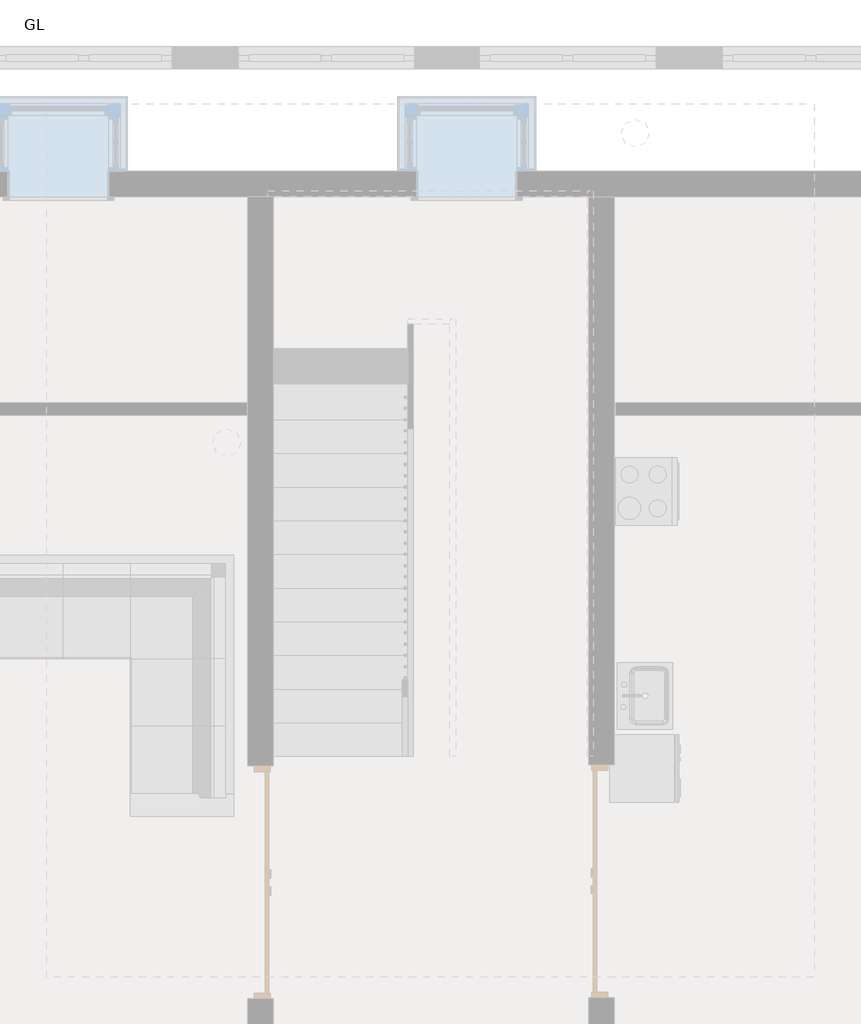
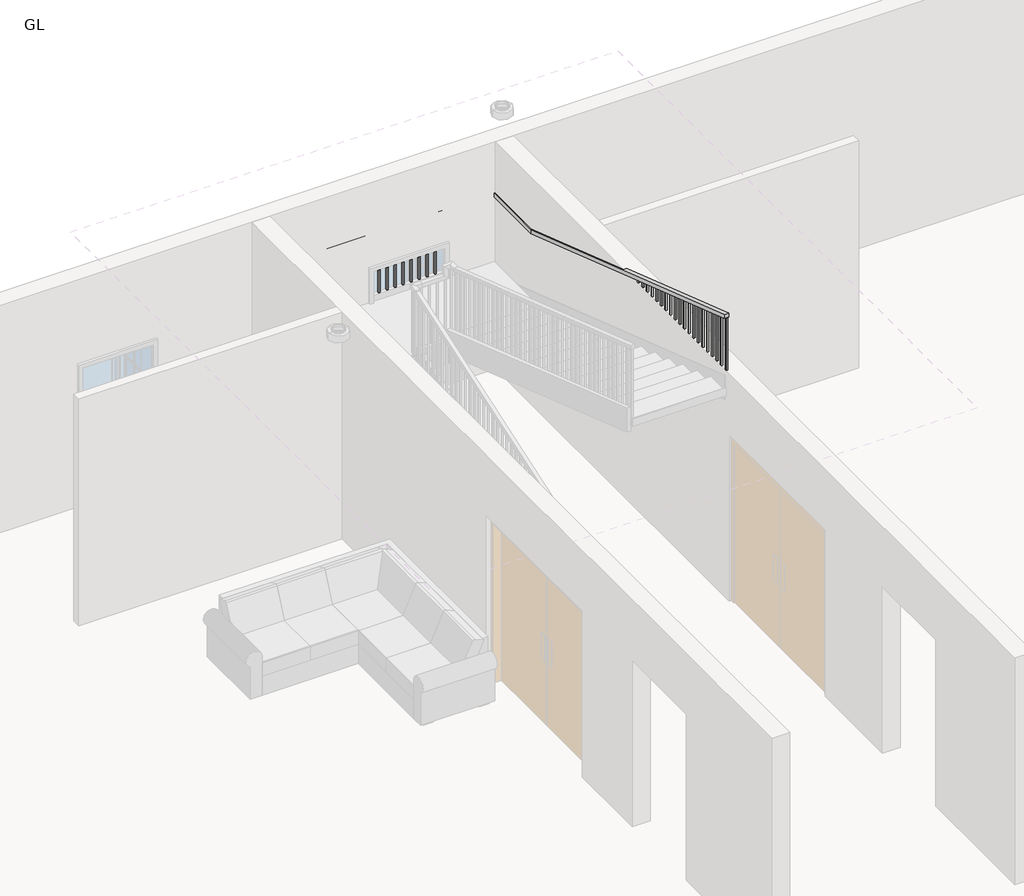
# One storey, part 3 of 5: 1 railing.
"""IFC4 building model written with IfcOpenShell, lengths in millimetres."""

from ifc_helpers import new_model, si_unit, frame, origin, place, context, project, spatial, polyline, outline, extrude, faceted_brep, element, save

model = new_model("IFC4")

# Units and contexts
model_context = context("Model", 3, world=origin())
ifc_project = project(units=[si_unit("LENGTHUNIT", "METRE", prefix="MILLI")], contexts=[model_context])

# Site, building, storey
site = spatial("IfcSite", under=ifc_project)
building = spatial("IfcBuilding", under=site)
storey = spatial("IfcBuildingStorey", under=building, Name="GL", Elevation=0.0)

# Railing
placement = place(None, origin())
element("IfcRailing", 1, ObjectType="Handrail - Rectangular", at=placement, inside=storey, context=model_context, shape_type="SolidModel", body=[
    faceted_brep([(-1899.5987998, 2564.5067329, 1017.8142857), (-1899.5987998, 2564.5067329, 964.1699957), (-1848.7987998, 2564.5067329, 964.1699957), (-1848.7987998, 2564.5067329, 1017.8142857), (-1899.5987998, 6526.9067329, 2362.2), (-1899.5987998, 6535.2899033, 2311.4), (-1848.7987998, 6535.2899033, 2311.4), (-1848.7987998, 6526.9067329, 2362.2), (-1899.5987998, 7682.6067329, 2311.4), (-1899.5987998, 7682.6067329, 2362.2), (1046.8012002, 7682.6067329, 2362.2), (1046.8012002, 7682.6067329, 2311.4), (-1848.7987998, 7631.8067329, 2311.4), (996.0012002, 7631.8067329, 2311.4), (-1848.7987998, 7631.8067329, 2362.2), (996.0012002, 7631.8067329, 2362.2), (1046.8012002, 6831.7067329, 2362.2), (1046.8012002, 6823.3235624, 2311.4), (996.0012002, 6823.3235624, 2311.4), (996.0012002, 6831.7067329, 2362.2), (1046.8012002, 2564.5067329, 3810.0), (996.0012002, 2564.5067329, 3810.0), (996.0012002, 2564.5067329, 3756.35571), (1046.8012002, 2564.5067329, 3756.35571)], [[[0, 1, 2, 3]], [[1, 0, 4, 5]], [[2, 1, 5, 6]], [[3, 2, 6, 7]], [[0, 3, 7, 4]], [[8, 9, 10, 11]], [[12, 8, 11, 13]], [[14, 12, 13, 15]], [[9, 14, 15, 10]], [[11, 10, 16, 17]], [[13, 11, 17, 18]], [[15, 13, 18, 19]], [[10, 15, 19, 16]], [[5, 4, 9, 8]], [[6, 5, 8, 12]], [[7, 6, 12, 14]], [[4, 7, 14, 9]], [[20, 21, 22, 23]], [[17, 16, 20, 23]], [[18, 17, 23, 22]], [[19, 18, 22, 21]], [[16, 19, 21, 20]]]),
    extrude(outline(polyline([(2586.7317329, 3748.815085), (2586.7317329, 2977.8831452), (2567.6817329, 2984.3465381), (2567.6817329, 3755.2784779), (2586.7317329, 3748.815085)])), frame((1011.8762002, 0.0, 0.0), z_axis=(1.0, 0.0, 0.0), x_axis=(0.0, 1.0, 0.0)), (0.0, 0.0, 1.0), 19.05),
    extrude(outline(polyline([(2688.3317329, 3714.3436565), (2688.3317329, 2943.4117167), (2669.2817329, 2949.8751095), (2669.2817329, 3720.8070493), (2688.3317329, 3714.3436565)])), frame((1011.8762002, 0.0, 0.0), z_axis=(1.0, 0.0, 0.0), x_axis=(0.0, 1.0, 0.0)), (0.0, 0.0, 1.0), 19.05),
    extrude(outline(polyline([(2789.9317329, 3679.8722279), (2789.9317329, 2908.9402881), (2770.8817329, 2915.403681), (2770.8817329, 3686.3356207), (2789.9317329, 3679.8722279)])), frame((1011.8762002, 0.0, 0.0), z_axis=(1.0, 0.0, 0.0), x_axis=(0.0, 1.0, 0.0)), (0.0, 0.0, 1.0), 19.05),
    extrude(outline(polyline([(2891.5317329, 3645.4007993), (2891.5317329, 2874.4688595), (2872.4817329, 2880.9322524), (2872.4817329, 3651.8641922), (2891.5317329, 3645.4007993)])), frame((1011.8762002, 0.0, 0.0), z_axis=(1.0, 0.0, 0.0), x_axis=(0.0, 1.0, 0.0)), (0.0, 0.0, 1.0), 19.05),
    extrude(outline(polyline([(2993.1317329, 3610.9293707), (2993.1317329, 2839.997431), (2974.0817329, 2846.4608238), (2974.0817329, 3617.3927636), (2993.1317329, 3610.9293707)])), frame((1011.8762002, 0.0, 0.0), z_axis=(1.0, 0.0, 0.0), x_axis=(0.0, 1.0, 0.0)), (0.0, 0.0, 1.0), 19.05),
    extrude(outline(polyline([(3094.7317329, 3576.4579422), (3094.7317329, 2805.5260024), (3075.6817329, 2811.9893952), (3075.6817329, 3582.921335), (3094.7317329, 3576.4579422)])), frame((1011.8762002, 0.0, 0.0), z_axis=(1.0, 0.0, 0.0), x_axis=(0.0, 1.0, 0.0)), (0.0, 0.0, 1.0), 19.05),
    extrude(outline(polyline([(3196.3317329, 3541.9865136), (3196.3317329, 2771.0545738), (3177.2817329, 2777.5179667), (3177.2817329, 3548.4499065), (3196.3317329, 3541.9865136)])), frame((1011.8762002, 0.0, 0.0), z_axis=(1.0, 0.0, 0.0), x_axis=(0.0, 1.0, 0.0)), (0.0, 0.0, 1.0), 19.05),
    extrude(outline(polyline([(3297.9317329, 3507.515085), (3297.9317329, 2736.5831452), (3278.8817329, 2743.0465381), (3278.8817329, 3513.9784779), (3297.9317329, 3507.515085)])), frame((1011.8762002, 0.0, 0.0), z_axis=(1.0, 0.0, 0.0), x_axis=(0.0, 1.0, 0.0)), (0.0, 0.0, 1.0), 19.05),
    extrude(outline(polyline([(3399.5317329, 3473.0436565), (3399.5317329, 2702.1117167), (3380.4817329, 2708.5751095), (3380.4817329, 3479.5070493), (3399.5317329, 3473.0436565)])), frame((1011.8762002, 0.0, 0.0), z_axis=(1.0, 0.0, 0.0), x_axis=(0.0, 1.0, 0.0)), (0.0, 0.0, 1.0), 19.05),
    extrude(outline(polyline([(3501.1317329, 3438.5722279), (3501.1317329, 2667.6402881), (3482.0817329, 2674.103681), (3482.0817329, 3445.0356207), (3501.1317329, 3438.5722279)])), frame((1011.8762002, 0.0, 0.0), z_axis=(1.0, 0.0, 0.0), x_axis=(0.0, 1.0, 0.0)), (0.0, 0.0, 1.0), 19.05),
    extrude(outline(polyline([(3602.7317329, 3404.1007993), (3602.7317329, 2633.1688595), (3583.6817329, 2639.6322524), (3583.6817329, 3410.5641922), (3602.7317329, 3404.1007993)])), frame((1011.8762002, 0.0, 0.0), z_axis=(1.0, 0.0, 0.0), x_axis=(0.0, 1.0, 0.0)), (0.0, 0.0, 1.0), 19.05),
    extrude(outline(polyline([(3704.3317329, 3369.6293707), (3704.3317329, 2598.697431), (3685.2817329, 2605.1608238), (3685.2817329, 3376.0927636), (3704.3317329, 3369.6293707)])), frame((1011.8762002, 0.0, 0.0), z_axis=(1.0, 0.0, 0.0), x_axis=(0.0, 1.0, 0.0)), (0.0, 0.0, 1.0), 19.05),
    extrude(outline(polyline([(3805.9317329, 3335.1579422), (3805.9317329, 2564.2260024), (3786.8817329, 2570.6893952), (3786.8817329, 3341.621335), (3805.9317329, 3335.1579422)])), frame((1011.8762002, 0.0, 0.0), z_axis=(1.0, 0.0, 0.0), x_axis=(0.0, 1.0, 0.0)), (0.0, 0.0, 1.0), 19.05),
    extrude(outline(polyline([(3907.5317329, 3300.6865136), (3907.5317329, 2529.7545738), (3888.4817329, 2536.2179667), (3888.4817329, 3307.1499065), (3907.5317329, 3300.6865136)])), frame((1011.8762002, 0.0, 0.0), z_axis=(1.0, 0.0, 0.0), x_axis=(0.0, 1.0, 0.0)), (0.0, 0.0, 1.0), 19.05),
    extrude(outline(polyline([(4009.1317329, 3266.215085), (4009.1317329, 2495.2831452), (3990.0817329, 2501.7465381), (3990.0817329, 3272.6784779), (4009.1317329, 3266.215085)])), frame((1011.8762002, 0.0, 0.0), z_axis=(1.0, 0.0, 0.0), x_axis=(0.0, 1.0, 0.0)), (0.0, 0.0, 1.0), 19.05),
    extrude(outline(polyline([(4110.7317329, 3231.7436565), (4110.7317329, 2460.8117167), (4091.6817329, 2467.2751095), (4091.6817329, 3238.2070493), (4110.7317329, 3231.7436565)])), frame((1011.8762002, 0.0, 0.0), z_axis=(1.0, 0.0, 0.0), x_axis=(0.0, 1.0, 0.0)), (0.0, 0.0, 1.0), 19.05),
    extrude(outline(polyline([(4212.3317329, 3197.2722279), (4212.3317329, 2426.3402881), (4193.2817329, 2432.803681), (4193.2817329, 3203.7356207), (4212.3317329, 3197.2722279)])), frame((1011.8762002, 0.0, 0.0), z_axis=(1.0, 0.0, 0.0), x_axis=(0.0, 1.0, 0.0)), (0.0, 0.0, 1.0), 19.05),
    extrude(outline(polyline([(4313.9317329, 3162.8007993), (4313.9317329, 2391.8688595), (4294.8817329, 2398.3322524), (4294.8817329, 3169.2641922), (4313.9317329, 3162.8007993)])), frame((1011.8762002, 0.0, 0.0), z_axis=(1.0, 0.0, 0.0), x_axis=(0.0, 1.0, 0.0)), (0.0, 0.0, 1.0), 19.05),
    extrude(outline(polyline([(4415.5317329, 3128.3293707), (4415.5317329, 2357.397431), (4396.4817329, 2363.8608238), (4396.4817329, 3134.7927636), (4415.5317329, 3128.3293707)])), frame((1011.8762002, 0.0, 0.0), z_axis=(1.0, 0.0, 0.0), x_axis=(0.0, 1.0, 0.0)), (0.0, 0.0, 1.0), 19.05),
    extrude(outline(polyline([(4517.1317329, 3093.8579422), (4517.1317329, 2322.9260024), (4498.0817329, 2329.3893952), (4498.0817329, 3100.321335), (4517.1317329, 3093.8579422)])), frame((1011.8762002, 0.0, 0.0), z_axis=(1.0, 0.0, 0.0), x_axis=(0.0, 1.0, 0.0)), (0.0, 0.0, 1.0), 19.05),
    extrude(outline(polyline([(4618.7317329, 3059.3865136), (4618.7317329, 2288.4545738), (4599.6817329, 2294.9179667), (4599.6817329, 3065.8499065), (4618.7317329, 3059.3865136)])), frame((1011.8762002, 0.0, 0.0), z_axis=(1.0, 0.0, 0.0), x_axis=(0.0, 1.0, 0.0)), (0.0, 0.0, 1.0), 19.05),
    extrude(outline(polyline([(4720.3317329, 3024.915085), (4720.3317329, 2253.9831452), (4701.2817329, 2260.4465381), (4701.2817329, 3031.3784779), (4720.3317329, 3024.915085)])), frame((1011.8762002, 0.0, 0.0), z_axis=(1.0, 0.0, 0.0), x_axis=(0.0, 1.0, 0.0)), (0.0, 0.0, 1.0), 19.05),
    extrude(outline(polyline([(4821.9317329, 2990.4436565), (4821.9317329, 2219.5117167), (4802.8817329, 2225.9751095), (4802.8817329, 2996.9070493), (4821.9317329, 2990.4436565)])), frame((1011.8762002, 0.0, 0.0), z_axis=(1.0, 0.0, 0.0), x_axis=(0.0, 1.0, 0.0)), (0.0, 0.0, 1.0), 19.05),
    extrude(outline(polyline([(4923.5317329, 2955.9722279), (4923.5317329, 2185.0402881), (4904.4817329, 2191.503681), (4904.4817329, 2962.4356207), (4923.5317329, 2955.9722279)])), frame((1011.8762002, 0.0, 0.0), z_axis=(1.0, 0.0, 0.0), x_axis=(0.0, 1.0, 0.0)), (0.0, 0.0, 1.0), 19.05),
    extrude(outline(polyline([(5025.1317329, 2921.5007993), (5025.1317329, 2150.5688595), (5006.0817329, 2157.0322524), (5006.0817329, 2927.9641922), (5025.1317329, 2921.5007993)])), frame((1011.8762002, 0.0, 0.0), z_axis=(1.0, 0.0, 0.0), x_axis=(0.0, 1.0, 0.0)), (0.0, 0.0, 1.0), 19.05),
    extrude(outline(polyline([(5126.7317329, 2887.0293707), (5126.7317329, 2116.097431), (5107.6817329, 2122.5608238), (5107.6817329, 2893.4927636), (5126.7317329, 2887.0293707)])), frame((1011.8762002, 0.0, 0.0), z_axis=(1.0, 0.0, 0.0), x_axis=(0.0, 1.0, 0.0)), (0.0, 0.0, 1.0), 19.05),
    extrude(outline(polyline([(5228.3317329, 2852.5579422), (5228.3317329, 2081.6260024), (5209.2817329, 2088.0893952), (5209.2817329, 2859.021335), (5228.3317329, 2852.5579422)])), frame((1011.8762002, 0.0, 0.0), z_axis=(1.0, 0.0, 0.0), x_axis=(0.0, 1.0, 0.0)), (0.0, 0.0, 1.0), 19.05),
    extrude(outline(polyline([(5329.9317329, 2818.0865136), (5329.9317329, 2047.1545738), (5310.8817329, 2053.6179667), (5310.8817329, 2824.5499065), (5329.9317329, 2818.0865136)])), frame((1011.8762002, 0.0, 0.0), z_axis=(1.0, 0.0, 0.0), x_axis=(0.0, 1.0, 0.0)), (0.0, 0.0, 1.0), 19.05),
    extrude(outline(polyline([(5431.5317329, 2783.615085), (5431.5317329, 2012.6831452), (5412.4817329, 2019.1465381), (5412.4817329, 2790.0784779), (5431.5317329, 2783.615085)])), frame((1011.8762002, 0.0, 0.0), z_axis=(1.0, 0.0, 0.0), x_axis=(0.0, 1.0, 0.0)), (0.0, 0.0, 1.0), 19.05),
    extrude(outline(polyline([(5533.1317329, 2749.1436565), (5533.1317329, 1978.2117167), (5514.0817329, 1984.6751095), (5514.0817329, 2755.6070493), (5533.1317329, 2749.1436565)])), frame((1011.8762002, 0.0, 0.0), z_axis=(1.0, 0.0, 0.0), x_axis=(0.0, 1.0, 0.0)), (0.0, 0.0, 1.0), 19.05),
    extrude(outline(polyline([(5634.7317329, 2714.6722279), (5634.7317329, 1943.7402881), (5615.6817329, 1950.203681), (5615.6817329, 2721.1356207), (5634.7317329, 2714.6722279)])), frame((1011.8762002, 0.0, 0.0), z_axis=(1.0, 0.0, 0.0), x_axis=(0.0, 1.0, 0.0)), (0.0, 0.0, 1.0), 19.05),
    extrude(outline(polyline([(5736.3317329, 2680.2007993), (5736.3317329, 1909.2688595), (5717.2817329, 1915.7322524), (5717.2817329, 2686.6641922), (5736.3317329, 2680.2007993)])), frame((1011.8762002, 0.0, 0.0), z_axis=(1.0, 0.0, 0.0), x_axis=(0.0, 1.0, 0.0)), (0.0, 0.0, 1.0), 19.05),
    extrude(outline(polyline([(5837.9317329, 2645.7293707), (5837.9317329, 1874.797431), (5818.8817329, 1881.2608238), (5818.8817329, 2652.1927636), (5837.9317329, 2645.7293707)])), frame((1011.8762002, 0.0, 0.0), z_axis=(1.0, 0.0, 0.0), x_axis=(0.0, 1.0, 0.0)), (0.0, 0.0, 1.0), 19.05),
    extrude(outline(polyline([(5939.5317329, 2611.2579422), (5939.5317329, 1840.3260024), (5920.4817329, 1846.7893952), (5920.4817329, 2617.721335), (5939.5317329, 2611.2579422)])), frame((1011.8762002, 0.0, 0.0), z_axis=(1.0, 0.0, 0.0), x_axis=(0.0, 1.0, 0.0)), (0.0, 0.0, 1.0), 19.05),
    extrude(outline(polyline([(6041.1317329, 2576.7865136), (6041.1317329, 1805.8545738), (6022.0817329, 1812.3179667), (6022.0817329, 2583.2499065), (6041.1317329, 2576.7865136)])), frame((1011.8762002, 0.0, 0.0), z_axis=(1.0, 0.0, 0.0), x_axis=(0.0, 1.0, 0.0)), (0.0, 0.0, 1.0), 19.05),
    extrude(outline(polyline([(6142.7317329, 2542.315085), (6142.7317329, 1771.3831452), (6123.6817329, 1777.8465381), (6123.6817329, 2548.7784779), (6142.7317329, 2542.315085)])), frame((1011.8762002, 0.0, 0.0), z_axis=(1.0, 0.0, 0.0), x_axis=(0.0, 1.0, 0.0)), (0.0, 0.0, 1.0), 19.05),
    extrude(outline(polyline([(6244.3317329, 2507.8436565), (6244.3317329, 1736.9117167), (6225.2817329, 1743.3751095), (6225.2817329, 2514.3070493), (6244.3317329, 2507.8436565)])), frame((1011.8762002, 0.0, 0.0), z_axis=(1.0, 0.0, 0.0), x_axis=(0.0, 1.0, 0.0)), (0.0, 0.0, 1.0), 19.05),
    extrude(outline(polyline([(6345.9317329, 2473.3722279), (6345.9317329, 1702.4402881), (6326.8817329, 1708.903681), (6326.8817329, 2479.8356207), (6345.9317329, 2473.3722279)])), frame((1011.8762002, 0.0, 0.0), z_axis=(1.0, 0.0, 0.0), x_axis=(0.0, 1.0, 0.0)), (0.0, 0.0, 1.0), 19.05),
    extrude(outline(polyline([(6447.5317329, 2438.9007993), (6447.5317329, 1667.9688595), (6428.4817329, 1674.4322524), (6428.4817329, 2445.3641922), (6447.5317329, 2438.9007993)])), frame((1011.8762002, 0.0, 0.0), z_axis=(1.0, 0.0, 0.0), x_axis=(0.0, 1.0, 0.0)), (0.0, 0.0, 1.0), 19.05),
    extrude(outline(polyline([(6549.1317329, 2404.4293707), (6549.1317329, 1633.497431), (6530.0817329, 1639.9608238), (6530.0817329, 2410.8927636), (6549.1317329, 2404.4293707)])), frame((1011.8762002, 0.0, 0.0), z_axis=(1.0, 0.0, 0.0), x_axis=(0.0, 1.0, 0.0)), (0.0, 0.0, 1.0), 19.05),
    extrude(outline(polyline([(6650.7317329, 2369.9579422), (6650.7317329, 1599.0260024), (6631.6817329, 1605.4893952), (6631.6817329, 2376.421335), (6650.7317329, 2369.9579422)])), frame((1011.8762002, 0.0, 0.0), z_axis=(1.0, 0.0, 0.0), x_axis=(0.0, 1.0, 0.0)), (0.0, 0.0, 1.0), 19.05),
    extrude(outline(polyline([(6752.3317329, 2335.4865136), (6752.3317329, 1564.5545738), (6733.2817329, 1571.0179667), (6733.2817329, 2341.9499065), (6752.3317329, 2335.4865136)])), frame((1011.8762002, 0.0, 0.0), z_axis=(1.0, 0.0, 0.0), x_axis=(0.0, 1.0, 0.0)), (0.0, 0.0, 1.0), 19.05),
    extrude(outline(polyline([(6853.9317329, 2311.4), (6853.9317329, 1530.0831452), (6834.8817329, 1536.5465381), (6834.8817329, 2311.4), (6853.9317329, 2311.4)])), frame((1011.8762002, 0.0, 0.0), z_axis=(1.0, 0.0, 0.0), x_axis=(0.0, 1.0, 0.0)), (0.0, 0.0, 1.0), 19.05),
    extrude(outline(polyline([(6955.5317329, 2311.4), (6955.5317329, 1495.6117167), (6936.4817329, 1502.0751095), (6936.4817329, 2311.4), (6955.5317329, 2311.4)])), frame((1011.8762002, 0.0, 0.0), z_axis=(1.0, 0.0, 0.0), x_axis=(0.0, 1.0, 0.0)), (0.0, 0.0, 1.0), 19.05),
    extrude(outline(polyline([(7057.1317329, 2311.4), (7057.1317329, 1461.1402881), (7038.0817329, 1467.603681), (7038.0817329, 2311.4), (7057.1317329, 2311.4)])), frame((1011.8762002, 0.0, 0.0), z_axis=(1.0, 0.0, 0.0), x_axis=(0.0, 1.0, 0.0)), (0.0, 0.0, 1.0), 19.05),
    extrude(outline(polyline([(7158.7317329, 2311.4), (7158.7317329, 1426.6688595), (7139.6817329, 1433.1322524), (7139.6817329, 2311.4), (7158.7317329, 2311.4)])), frame((1011.8762002, 0.0, 0.0), z_axis=(1.0, 0.0, 0.0), x_axis=(0.0, 1.0, 0.0)), (0.0, 0.0, 1.0), 19.05),
    extrude(outline(polyline([(7260.3317329, 2311.4), (7260.3317329, 1392.197431), (7241.2817329, 1398.6608238), (7241.2817329, 2311.4), (7260.3317329, 2311.4)])), frame((1011.8762002, 0.0, 0.0), z_axis=(1.0, 0.0, 0.0), x_axis=(0.0, 1.0, 0.0)), (0.0, 0.0, 1.0), 19.05),
    extrude(outline(polyline([(7361.9317329, 2311.4), (7361.9317329, 1357.7260024), (7342.8817329, 1364.1893952), (7342.8817329, 2311.4), (7361.9317329, 2311.4)])), frame((1011.8762002, 0.0, 0.0), z_axis=(1.0, 0.0, 0.0), x_axis=(0.0, 1.0, 0.0)), (0.0, 0.0, 1.0), 19.05),
    extrude(outline(polyline([(7463.5317329, 2311.4), (7463.5317329, 1323.2545738), (7444.4817329, 1329.7179667), (7444.4817329, 2311.4), (7463.5317329, 2311.4)])), frame((1011.8762002, 0.0, 0.0), z_axis=(1.0, 0.0, 0.0), x_axis=(0.0, 1.0, 0.0)), (0.0, 0.0, 1.0), 19.05),
    extrude(outline(polyline([(7565.1317329, 2311.4), (7565.1317329, 1288.7831452), (7546.0817329, 1295.2465381), (7546.0817329, 2311.4), (7565.1317329, 2311.4)])), frame((1011.8762002, 0.0, 0.0), z_axis=(1.0, 0.0, 0.0), x_axis=(0.0, 1.0, 0.0)), (0.0, 0.0, 1.0), 19.05),
    extrude(outline(polyline([(961.0762002, 7666.7317329), (980.1262002, 7666.7317329), (980.1262002, 7647.6817329), (961.0762002, 7647.6817329), (961.0762002, 7666.7317329)])), frame((0.0, 0.0, 1524.0), z_axis=(0.0, 0.0, 1.0), x_axis=(1.0, 0.0, 0.0)), (0.0, 0.0, 1.0), 787.4),
    extrude(outline(polyline([(859.4762002, 7666.7317329), (878.5262002, 7666.7317329), (878.5262002, 7647.6817329), (859.4762002, 7647.6817329), (859.4762002, 7666.7317329)])), frame((0.0, 0.0, 1524.0), z_axis=(0.0, 0.0, 1.0), x_axis=(1.0, 0.0, 0.0)), (0.0, 0.0, 1.0), 787.4),
    extrude(outline(polyline([(757.8762002, 7666.7317329), (776.9262002, 7666.7317329), (776.9262002, 7647.6817329), (757.8762002, 7647.6817329), (757.8762002, 7666.7317329)])), frame((0.0, 0.0, 1524.0), z_axis=(0.0, 0.0, 1.0), x_axis=(1.0, 0.0, 0.0)), (0.0, 0.0, 1.0), 787.4),
    extrude(outline(polyline([(656.2762002, 7666.7317329), (675.3262002, 7666.7317329), (675.3262002, 7647.6817329), (656.2762002, 7647.6817329), (656.2762002, 7666.7317329)])), frame((0.0, 0.0, 1524.0), z_axis=(0.0, 0.0, 1.0), x_axis=(1.0, 0.0, 0.0)), (0.0, 0.0, 1.0), 787.4),
    extrude(outline(polyline([(554.6762002, 7666.7317329), (573.7262002, 7666.7317329), (573.7262002, 7647.6817329), (554.6762002, 7647.6817329), (554.6762002, 7666.7317329)])), frame((0.0, 0.0, 1524.0), z_axis=(0.0, 0.0, 1.0), x_axis=(1.0, 0.0, 0.0)), (0.0, 0.0, 1.0), 787.4),
    extrude(outline(polyline([(453.0762002, 7666.7317329), (472.1262002, 7666.7317329), (472.1262002, 7647.6817329), (453.0762002, 7647.6817329), (453.0762002, 7666.7317329)])), frame((0.0, 0.0, 1524.0), z_axis=(0.0, 0.0, 1.0), x_axis=(1.0, 0.0, 0.0)), (0.0, 0.0, 1.0), 787.4),
    extrude(outline(polyline([(351.4762002, 7666.7317329), (370.5262002, 7666.7317329), (370.5262002, 7647.6817329), (351.4762002, 7647.6817329), (351.4762002, 7666.7317329)])), frame((0.0, 0.0, 1524.0), z_axis=(0.0, 0.0, 1.0), x_axis=(1.0, 0.0, 0.0)), (0.0, 0.0, 1.0), 787.4),
    extrude(outline(polyline([(249.8762002, 7666.7317329), (268.9262002, 7666.7317329), (268.9262002, 7647.6817329), (249.8762002, 7647.6817329), (249.8762002, 7666.7317329)])), frame((0.0, 0.0, 1524.0), z_axis=(0.0, 0.0, 1.0), x_axis=(1.0, 0.0, 0.0)), (0.0, 0.0, 1.0), 787.4),
    extrude(outline(polyline([(148.2762002, 7666.7317329), (167.3262002, 7666.7317329), (167.3262002, 7647.6817329), (148.2762002, 7647.6817329), (148.2762002, 7666.7317329)])), frame((0.0, 0.0, 1524.0), z_axis=(0.0, 0.0, 1.0), x_axis=(1.0, 0.0, 0.0)), (0.0, 0.0, 1.0), 787.4),
    extrude(outline(polyline([(46.6762002, 7666.7317329), (65.7262002, 7666.7317329), (65.7262002, 7647.6817329), (46.6762002, 7647.6817329), (46.6762002, 7666.7317329)])), frame((0.0, 0.0, 1524.0), z_axis=(0.0, 0.0, 1.0), x_axis=(1.0, 0.0, 0.0)), (0.0, 0.0, 1.0), 787.4),
    extrude(outline(polyline([(-54.9237998, 7666.7317329), (-35.8737998, 7666.7317329), (-35.8737998, 7647.6817329), (-54.9237998, 7647.6817329), (-54.9237998, 7666.7317329)])), frame((0.0, 0.0, 1524.0), z_axis=(0.0, 0.0, 1.0), x_axis=(1.0, 0.0, 0.0)), (0.0, 0.0, 1.0), 787.4),
    extrude(outline(polyline([(-156.5237998, 7666.7317329), (-137.4737998, 7666.7317329), (-137.4737998, 7647.6817329), (-156.5237998, 7647.6817329), (-156.5237998, 7666.7317329)])), frame((0.0, 0.0, 1524.0), z_axis=(0.0, 0.0, 1.0), x_axis=(1.0, 0.0, 0.0)), (0.0, 0.0, 1.0), 787.4),
    extrude(outline(polyline([(-258.1237998, 7666.7317329), (-239.0737998, 7666.7317329), (-239.0737998, 7647.6817329), (-258.1237998, 7647.6817329), (-258.1237998, 7666.7317329)])), frame((0.0, 0.0, 1524.0), z_axis=(0.0, 0.0, 1.0), x_axis=(1.0, 0.0, 0.0)), (0.0, 0.0, 1.0), 787.4),
    extrude(outline(polyline([(-359.7237998, 7666.7317329), (-340.6737998, 7666.7317329), (-340.6737998, 7647.6817329), (-359.7237998, 7647.6817329), (-359.7237998, 7666.7317329)])), frame((0.0, 0.0, 1524.0), z_axis=(0.0, 0.0, 1.0), x_axis=(1.0, 0.0, 0.0)), (0.0, 0.0, 1.0), 787.4),
    extrude(outline(polyline([(-461.3237998, 7666.7317329), (-442.2737998, 7666.7317329), (-442.2737998, 7647.6817329), (-461.3237998, 7647.6817329), (-461.3237998, 7666.7317329)])), frame((0.0, 0.0, 1524.0), z_axis=(0.0, 0.0, 1.0), x_axis=(1.0, 0.0, 0.0)), (0.0, 0.0, 1.0), 787.4),
    extrude(outline(polyline([(-562.9237998, 7666.7317329), (-543.8737998, 7666.7317329), (-543.8737998, 7647.6817329), (-562.9237998, 7647.6817329), (-562.9237998, 7666.7317329)])), frame((0.0, 0.0, 1524.0), z_axis=(0.0, 0.0, 1.0), x_axis=(1.0, 0.0, 0.0)), (0.0, 0.0, 1.0), 787.4),
    extrude(outline(polyline([(-664.5237998, 7666.7317329), (-645.4737998, 7666.7317329), (-645.4737998, 7647.6817329), (-664.5237998, 7647.6817329), (-664.5237998, 7666.7317329)])), frame((0.0, 0.0, 1524.0), z_axis=(0.0, 0.0, 1.0), x_axis=(1.0, 0.0, 0.0)), (0.0, 0.0, 1.0), 787.4),
    extrude(outline(polyline([(-766.1237998, 7666.7317329), (-747.0737998, 7666.7317329), (-747.0737998, 7647.6817329), (-766.1237998, 7647.6817329), (-766.1237998, 7666.7317329)])), frame((0.0, 0.0, 1524.0), z_axis=(0.0, 0.0, 1.0), x_axis=(1.0, 0.0, 0.0)), (0.0, 0.0, 1.0), 787.4),
    extrude(outline(polyline([(-867.7237998, 7666.7317329), (-848.6737998, 7666.7317329), (-848.6737998, 7647.6817329), (-867.7237998, 7647.6817329), (-867.7237998, 7666.7317329)])), frame((0.0, 0.0, 1524.0), z_axis=(0.0, 0.0, 1.0), x_axis=(1.0, 0.0, 0.0)), (0.0, 0.0, 1.0), 787.4),
    extrude(outline(polyline([(-969.3237998, 7666.7317329), (-950.2737998, 7666.7317329), (-950.2737998, 7647.6817329), (-969.3237998, 7647.6817329), (-969.3237998, 7666.7317329)])), frame((0.0, 0.0, 1524.0), z_axis=(0.0, 0.0, 1.0), x_axis=(1.0, 0.0, 0.0)), (0.0, 0.0, 1.0), 787.4),
    extrude(outline(polyline([(-1070.9237998, 7666.7317329), (-1051.8737998, 7666.7317329), (-1051.8737998, 7647.6817329), (-1070.9237998, 7647.6817329), (-1070.9237998, 7666.7317329)])), frame((0.0, 0.0, 1524.0), z_axis=(0.0, 0.0, 1.0), x_axis=(1.0, 0.0, 0.0)), (0.0, 0.0, 1.0), 787.4),
    extrude(outline(polyline([(-1172.5237998, 7666.7317329), (-1153.4737998, 7666.7317329), (-1153.4737998, 7647.6817329), (-1172.5237998, 7647.6817329), (-1172.5237998, 7666.7317329)])), frame((0.0, 0.0, 1524.0), z_axis=(0.0, 0.0, 1.0), x_axis=(1.0, 0.0, 0.0)), (0.0, 0.0, 1.0), 787.4),
    extrude(outline(polyline([(-1274.1237998, 7666.7317329), (-1255.0737998, 7666.7317329), (-1255.0737998, 7647.6817329), (-1274.1237998, 7647.6817329), (-1274.1237998, 7666.7317329)])), frame((0.0, 0.0, 1524.0), z_axis=(0.0, 0.0, 1.0), x_axis=(1.0, 0.0, 0.0)), (0.0, 0.0, 1.0), 787.4),
    extrude(outline(polyline([(-1375.7237998, 7666.7317329), (-1356.6737998, 7666.7317329), (-1356.6737998, 7647.6817329), (-1375.7237998, 7647.6817329), (-1375.7237998, 7666.7317329)])), frame((0.0, 0.0, 1524.0), z_axis=(0.0, 0.0, 1.0), x_axis=(1.0, 0.0, 0.0)), (0.0, 0.0, 1.0), 787.4),
    extrude(outline(polyline([(-1477.3237998, 7666.7317329), (-1458.2737998, 7666.7317329), (-1458.2737998, 7647.6817329), (-1477.3237998, 7647.6817329), (-1477.3237998, 7666.7317329)])), frame((0.0, 0.0, 1524.0), z_axis=(0.0, 0.0, 1.0), x_axis=(1.0, 0.0, 0.0)), (0.0, 0.0, 1.0), 787.4),
    extrude(outline(polyline([(-1578.9237998, 7666.7317329), (-1559.8737998, 7666.7317329), (-1559.8737998, 7647.6817329), (-1578.9237998, 7647.6817329), (-1578.9237998, 7666.7317329)])), frame((0.0, 0.0, 1524.0), z_axis=(0.0, 0.0, 1.0), x_axis=(1.0, 0.0, 0.0)), (0.0, 0.0, 1.0), 787.4),
    extrude(outline(polyline([(-1680.5237998, 7666.7317329), (-1661.4737998, 7666.7317329), (-1661.4737998, 7647.6817329), (-1680.5237998, 7647.6817329), (-1680.5237998, 7666.7317329)])), frame((0.0, 0.0, 1524.0), z_axis=(0.0, 0.0, 1.0), x_axis=(1.0, 0.0, 0.0)), (0.0, 0.0, 1.0), 787.4),
    extrude(outline(polyline([(-1782.1237998, 7666.7317329), (-1763.0737998, 7666.7317329), (-1763.0737998, 7647.6817329), (-1782.1237998, 7647.6817329), (-1782.1237998, 7666.7317329)])), frame((0.0, 0.0, 1524.0), z_axis=(0.0, 0.0, 1.0), x_axis=(1.0, 0.0, 0.0)), (0.0, 0.0, 1.0), 787.4),
    extrude(outline(polyline([(-1883.7237998, 7634.9817329), (-1883.7237998, 7654.0317329), (-1864.6737998, 7654.0317329), (-1864.6737998, 7634.9817329), (-1883.7237998, 7634.9817329)])), frame((0.0, 0.0, 1826.9857143), z_axis=(0.0, 0.0, 1.0), x_axis=(1.0, 0.0, 0.0)), (0.0, 0.0, 1.0), 484.4142857),
    extrude(outline(polyline([(-1883.7237998, 7533.3817329), (-1883.7237998, 7552.4317329), (-1864.6737998, 7552.4317329), (-1864.6737998, 7533.3817329), (-1883.7237998, 7533.3817329)])), frame((0.0, 0.0, 1792.5142857), z_axis=(0.0, 0.0, 1.0), x_axis=(1.0, 0.0, 0.0)), (0.0, 0.0, 1.0), 518.8857143),
    extrude(outline(polyline([(-1883.7237998, 7431.7817329), (-1883.7237998, 7450.8317329), (-1864.6737998, 7450.8317329), (-1864.6737998, 7431.7817329), (-1883.7237998, 7431.7817329)])), frame((0.0, 0.0, 1758.0428571), z_axis=(0.0, 0.0, 1.0), x_axis=(1.0, 0.0, 0.0)), (0.0, 0.0, 1.0), 553.3571429),
    extrude(outline(polyline([(-1883.7237998, 7330.1817329), (-1883.7237998, 7349.2317329), (-1864.6737998, 7349.2317329), (-1864.6737998, 7330.1817329), (-1883.7237998, 7330.1817329)])), frame((0.0, 0.0, 1723.5714286), z_axis=(0.0, 0.0, 1.0), x_axis=(1.0, 0.0, 0.0)), (0.0, 0.0, 1.0), 587.8285714),
    extrude(outline(polyline([(-1883.7237998, 7228.5817329), (-1883.7237998, 7247.6317329), (-1864.6737998, 7247.6317329), (-1864.6737998, 7228.5817329), (-1883.7237998, 7228.5817329)])), frame((0.0, 0.0, 1689.1), z_axis=(0.0, 0.0, 1.0), x_axis=(1.0, 0.0, 0.0)), (0.0, 0.0, 1.0), 622.3),
    extrude(outline(polyline([(-1883.7237998, 7126.9817329), (-1883.7237998, 7146.0317329), (-1864.6737998, 7146.0317329), (-1864.6737998, 7126.9817329), (-1883.7237998, 7126.9817329)])), frame((0.0, 0.0, 1654.6285714), z_axis=(0.0, 0.0, 1.0), x_axis=(1.0, 0.0, 0.0)), (0.0, 0.0, 1.0), 656.7714286),
    extrude(outline(polyline([(-1883.7237998, 7025.3817329), (-1883.7237998, 7044.4317329), (-1864.6737998, 7044.4317329), (-1864.6737998, 7025.3817329), (-1883.7237998, 7025.3817329)])), frame((0.0, 0.0, 1524.0), z_axis=(0.0, 0.0, 1.0), x_axis=(1.0, 0.0, 0.0)), (0.0, 0.0, 1.0), 787.4),
    extrude(outline(polyline([(-1883.7237998, 6923.7817329), (-1883.7237998, 6942.8317329), (-1864.6737998, 6942.8317329), (-1864.6737998, 6923.7817329), (-1883.7237998, 6923.7817329)])), frame((0.0, 0.0, 1524.0), z_axis=(0.0, 0.0, 1.0), x_axis=(1.0, 0.0, 0.0)), (0.0, 0.0, 1.0), 787.4),
    extrude(outline(polyline([(-1883.7237998, 6822.1817329), (-1883.7237998, 6841.2317329), (-1864.6737998, 6841.2317329), (-1864.6737998, 6822.1817329), (-1883.7237998, 6822.1817329)])), frame((0.0, 0.0, 1524.0), z_axis=(0.0, 0.0, 1.0), x_axis=(1.0, 0.0, 0.0)), (0.0, 0.0, 1.0), 787.4),
    extrude(outline(polyline([(-1883.7237998, 6720.5817329), (-1883.7237998, 6739.6317329), (-1864.6737998, 6739.6317329), (-1864.6737998, 6720.5817329), (-1883.7237998, 6720.5817329)])), frame((0.0, 0.0, 1524.0), z_axis=(0.0, 0.0, 1.0), x_axis=(1.0, 0.0, 0.0)), (0.0, 0.0, 1.0), 787.4),
    extrude(outline(polyline([(-1883.7237998, 6618.9817329), (-1883.7237998, 6638.0317329), (-1864.6737998, 6638.0317329), (-1864.6737998, 6618.9817329), (-1883.7237998, 6618.9817329)])), frame((0.0, 0.0, 1524.0), z_axis=(0.0, 0.0, 1.0), x_axis=(1.0, 0.0, 0.0)), (0.0, 0.0, 1.0), 787.4),
    extrude(outline(polyline([(6536.4317329, 2311.7874065), (6536.4317329, 1524.0), (6517.3817329, 1524.0), (6517.3817329, 2305.3240136), (6536.4317329, 2311.7874065)])), frame((-1883.7237998, 0.0, 0.0), z_axis=(1.0, 0.0, 0.0), x_axis=(0.0, 1.0, 0.0)), (0.0, 0.0, 1.0), 19.05),
    extrude(outline(polyline([(6434.8317329, 2277.3159779), (6434.8317329, 1506.3840381), (6415.7817329, 1499.9206452), (6415.7817329, 2270.852585), (6434.8317329, 2277.3159779)])), frame((-1883.7237998, 0.0, 0.0), z_axis=(1.0, 0.0, 0.0), x_axis=(0.0, 1.0, 0.0)), (0.0, 0.0, 1.0), 19.05),
    extrude(outline(polyline([(6333.2317329, 2242.8445493), (6333.2317329, 1471.9126095), (6314.1817329, 1465.4492167), (6314.1817329, 2236.3811565), (6333.2317329, 2242.8445493)])), frame((-1883.7237998, 0.0, 0.0), z_axis=(1.0, 0.0, 0.0), x_axis=(0.0, 1.0, 0.0)), (0.0, 0.0, 1.0), 19.05),
    extrude(outline(polyline([(6231.6317329, 2208.3731207), (6231.6317329, 1437.441181), (6212.5817329, 1430.9777881), (6212.5817329, 2201.9097279), (6231.6317329, 2208.3731207)])), frame((-1883.7237998, 0.0, 0.0), z_axis=(1.0, 0.0, 0.0), x_axis=(0.0, 1.0, 0.0)), (0.0, 0.0, 1.0), 19.05),
    extrude(outline(polyline([(6130.0317329, 2173.9016922), (6130.0317329, 1402.9697524), (6110.9817329, 1396.5063595), (6110.9817329, 2167.4382993), (6130.0317329, 2173.9016922)])), frame((-1883.7237998, 0.0, 0.0), z_axis=(1.0, 0.0, 0.0), x_axis=(0.0, 1.0, 0.0)), (0.0, 0.0, 1.0), 19.05),
    extrude(outline(polyline([(6028.4317329, 2139.4302636), (6028.4317329, 1368.4983238), (6009.3817329, 1362.034931), (6009.3817329, 2132.9668707), (6028.4317329, 2139.4302636)])), frame((-1883.7237998, 0.0, 0.0), z_axis=(1.0, 0.0, 0.0), x_axis=(0.0, 1.0, 0.0)), (0.0, 0.0, 1.0), 19.05),
    extrude(outline(polyline([(5926.8317329, 2104.958835), (5926.8317329, 1334.0268952), (5907.7817329, 1327.5635024), (5907.7817329, 2098.4954422), (5926.8317329, 2104.958835)])), frame((-1883.7237998, 0.0, 0.0), z_axis=(1.0, 0.0, 0.0), x_axis=(0.0, 1.0, 0.0)), (0.0, 0.0, 1.0), 19.05),
    extrude(outline(polyline([(5825.2317329, 2070.4874065), (5825.2317329, 1299.5554667), (5806.1817329, 1293.0920738), (5806.1817329, 2064.0240136), (5825.2317329, 2070.4874065)])), frame((-1883.7237998, 0.0, 0.0), z_axis=(1.0, 0.0, 0.0), x_axis=(0.0, 1.0, 0.0)), (0.0, 0.0, 1.0), 19.05),
    extrude(outline(polyline([(5723.6317329, 2036.0159779), (5723.6317329, 1265.0840381), (5704.5817329, 1258.6206452), (5704.5817329, 2029.552585), (5723.6317329, 2036.0159779)])), frame((-1883.7237998, 0.0, 0.0), z_axis=(1.0, 0.0, 0.0), x_axis=(0.0, 1.0, 0.0)), (0.0, 0.0, 1.0), 19.05),
    extrude(outline(polyline([(5622.0317329, 2001.5445493), (5622.0317329, 1230.6126095), (5602.9817329, 1224.1492167), (5602.9817329, 1995.0811565), (5622.0317329, 2001.5445493)])), frame((-1883.7237998, 0.0, 0.0), z_axis=(1.0, 0.0, 0.0), x_axis=(0.0, 1.0, 0.0)), (0.0, 0.0, 1.0), 19.05),
    extrude(outline(polyline([(5520.4317329, 1967.0731207), (5520.4317329, 1196.141181), (5501.3817329, 1189.6777881), (5501.3817329, 1960.6097279), (5520.4317329, 1967.0731207)])), frame((-1883.7237998, 0.0, 0.0), z_axis=(1.0, 0.0, 0.0), x_axis=(0.0, 1.0, 0.0)), (0.0, 0.0, 1.0), 19.05),
    extrude(outline(polyline([(5418.8317329, 1932.6016922), (5418.8317329, 1161.6697524), (5399.7817329, 1155.2063595), (5399.7817329, 1926.1382993), (5418.8317329, 1932.6016922)])), frame((-1883.7237998, 0.0, 0.0), z_axis=(1.0, 0.0, 0.0), x_axis=(0.0, 1.0, 0.0)), (0.0, 0.0, 1.0), 19.05),
    extrude(outline(polyline([(5317.2317329, 1898.1302636), (5317.2317329, 1127.1983238), (5298.1817329, 1120.734931), (5298.1817329, 1891.6668707), (5317.2317329, 1898.1302636)])), frame((-1883.7237998, 0.0, 0.0), z_axis=(1.0, 0.0, 0.0), x_axis=(0.0, 1.0, 0.0)), (0.0, 0.0, 1.0), 19.05),
    extrude(outline(polyline([(5215.6317329, 1863.658835), (5215.6317329, 1092.7268952), (5196.5817329, 1086.2635024), (5196.5817329, 1857.1954422), (5215.6317329, 1863.658835)])), frame((-1883.7237998, 0.0, 0.0), z_axis=(1.0, 0.0, 0.0), x_axis=(0.0, 1.0, 0.0)), (0.0, 0.0, 1.0), 19.05),
    extrude(outline(polyline([(5114.0317329, 1829.1874065), (5114.0317329, 1058.2554667), (5094.9817329, 1051.7920738), (5094.9817329, 1822.7240136), (5114.0317329, 1829.1874065)])), frame((-1883.7237998, 0.0, 0.0), z_axis=(1.0, 0.0, 0.0), x_axis=(0.0, 1.0, 0.0)), (0.0, 0.0, 1.0), 19.05),
    extrude(outline(polyline([(5012.4317329, 1794.7159779), (5012.4317329, 1023.7840381), (4993.3817329, 1017.3206452), (4993.3817329, 1788.252585), (5012.4317329, 1794.7159779)])), frame((-1883.7237998, 0.0, 0.0), z_axis=(1.0, 0.0, 0.0), x_axis=(0.0, 1.0, 0.0)), (0.0, 0.0, 1.0), 19.05),
    extrude(outline(polyline([(4910.8317329, 1760.2445493), (4910.8317329, 989.3126095), (4891.7817329, 982.8492167), (4891.7817329, 1753.7811565), (4910.8317329, 1760.2445493)])), frame((-1883.7237998, 0.0, 0.0), z_axis=(1.0, 0.0, 0.0), x_axis=(0.0, 1.0, 0.0)), (0.0, 0.0, 1.0), 19.05),
    extrude(outline(polyline([(4809.2317329, 1725.7731207), (4809.2317329, 954.841181), (4790.1817329, 948.3777881), (4790.1817329, 1719.3097279), (4809.2317329, 1725.7731207)])), frame((-1883.7237998, 0.0, 0.0), z_axis=(1.0, 0.0, 0.0), x_axis=(0.0, 1.0, 0.0)), (0.0, 0.0, 1.0), 19.05),
    extrude(outline(polyline([(4707.6317329, 1691.3016922), (4707.6317329, 920.3697524), (4688.5817329, 913.9063595), (4688.5817329, 1684.8382993), (4707.6317329, 1691.3016922)])), frame((-1883.7237998, 0.0, 0.0), z_axis=(1.0, 0.0, 0.0), x_axis=(0.0, 1.0, 0.0)), (0.0, 0.0, 1.0), 19.05),
    extrude(outline(polyline([(4606.0317329, 1656.8302636), (4606.0317329, 885.8983238), (4586.9817329, 879.434931), (4586.9817329, 1650.3668707), (4606.0317329, 1656.8302636)])), frame((-1883.7237998, 0.0, 0.0), z_axis=(1.0, 0.0, 0.0), x_axis=(0.0, 1.0, 0.0)), (0.0, 0.0, 1.0), 19.05),
    extrude(outline(polyline([(4504.4317329, 1622.358835), (4504.4317329, 851.4268952), (4485.3817329, 844.9635024), (4485.3817329, 1615.8954422), (4504.4317329, 1622.358835)])), frame((-1883.7237998, 0.0, 0.0), z_axis=(1.0, 0.0, 0.0), x_axis=(0.0, 1.0, 0.0)), (0.0, 0.0, 1.0), 19.05),
    extrude(outline(polyline([(4402.8317329, 1587.8874065), (4402.8317329, 816.9554667), (4383.7817329, 810.4920738), (4383.7817329, 1581.4240136), (4402.8317329, 1587.8874065)])), frame((-1883.7237998, 0.0, 0.0), z_axis=(1.0, 0.0, 0.0), x_axis=(0.0, 1.0, 0.0)), (0.0, 0.0, 1.0), 19.05),
    extrude(outline(polyline([(4301.2317329, 1553.4159779), (4301.2317329, 782.4840381), (4282.1817329, 776.0206452), (4282.1817329, 1546.952585), (4301.2317329, 1553.4159779)])), frame((-1883.7237998, 0.0, 0.0), z_axis=(1.0, 0.0, 0.0), x_axis=(0.0, 1.0, 0.0)), (0.0, 0.0, 1.0), 19.05),
    extrude(outline(polyline([(4199.6317329, 1518.9445493), (4199.6317329, 748.0126095), (4180.5817329, 741.5492167), (4180.5817329, 1512.4811565), (4199.6317329, 1518.9445493)])), frame((-1883.7237998, 0.0, 0.0), z_axis=(1.0, 0.0, 0.0), x_axis=(0.0, 1.0, 0.0)), (0.0, 0.0, 1.0), 19.05),
    extrude(outline(polyline([(4098.0317329, 1484.4731207), (4098.0317329, 713.541181), (4078.9817329, 707.0777881), (4078.9817329, 1478.0097279), (4098.0317329, 1484.4731207)])), frame((-1883.7237998, 0.0, 0.0), z_axis=(1.0, 0.0, 0.0), x_axis=(0.0, 1.0, 0.0)), (0.0, 0.0, 1.0), 19.05),
    extrude(outline(polyline([(3996.4317329, 1450.0016922), (3996.4317329, 679.0697524), (3977.3817329, 672.6063595), (3977.3817329, 1443.5382993), (3996.4317329, 1450.0016922)])), frame((-1883.7237998, 0.0, 0.0), z_axis=(1.0, 0.0, 0.0), x_axis=(0.0, 1.0, 0.0)), (0.0, 0.0, 1.0), 19.05),
    extrude(outline(polyline([(3894.8317329, 1415.5302636), (3894.8317329, 644.5983238), (3875.7817329, 638.134931), (3875.7817329, 1409.0668707), (3894.8317329, 1415.5302636)])), frame((-1883.7237998, 0.0, 0.0), z_axis=(1.0, 0.0, 0.0), x_axis=(0.0, 1.0, 0.0)), (0.0, 0.0, 1.0), 19.05),
    extrude(outline(polyline([(3793.2317329, 1381.058835), (3793.2317329, 610.1268952), (3774.1817329, 603.6635024), (3774.1817329, 1374.5954422), (3793.2317329, 1381.058835)])), frame((-1883.7237998, 0.0, 0.0), z_axis=(1.0, 0.0, 0.0), x_axis=(0.0, 1.0, 0.0)), (0.0, 0.0, 1.0), 19.05),
    extrude(outline(polyline([(3691.6317329, 1346.5874065), (3691.6317329, 575.6554667), (3672.5817329, 569.1920738), (3672.5817329, 1340.1240136), (3691.6317329, 1346.5874065)])), frame((-1883.7237998, 0.0, 0.0), z_axis=(1.0, 0.0, 0.0), x_axis=(0.0, 1.0, 0.0)), (0.0, 0.0, 1.0), 19.05),
    extrude(outline(polyline([(3590.0317329, 1312.1159779), (3590.0317329, 541.1840381), (3570.9817329, 534.7206452), (3570.9817329, 1305.652585), (3590.0317329, 1312.1159779)])), frame((-1883.7237998, 0.0, 0.0), z_axis=(1.0, 0.0, 0.0), x_axis=(0.0, 1.0, 0.0)), (0.0, 0.0, 1.0), 19.05),
    extrude(outline(polyline([(3488.4317329, 1277.6445493), (3488.4317329, 506.7126095), (3469.3817329, 500.2492167), (3469.3817329, 1271.1811565), (3488.4317329, 1277.6445493)])), frame((-1883.7237998, 0.0, 0.0), z_axis=(1.0, 0.0, 0.0), x_axis=(0.0, 1.0, 0.0)), (0.0, 0.0, 1.0), 19.05),
    extrude(outline(polyline([(3386.8317329, 1243.1731207), (3386.8317329, 472.241181), (3367.7817329, 465.7777881), (3367.7817329, 1236.7097279), (3386.8317329, 1243.1731207)])), frame((-1883.7237998, 0.0, 0.0), z_axis=(1.0, 0.0, 0.0), x_axis=(0.0, 1.0, 0.0)), (0.0, 0.0, 1.0), 19.05),
    extrude(outline(polyline([(3285.2317329, 1208.7016922), (3285.2317329, 437.7697524), (3266.1817329, 431.3063595), (3266.1817329, 1202.2382993), (3285.2317329, 1208.7016922)])), frame((-1883.7237998, 0.0, 0.0), z_axis=(1.0, 0.0, 0.0), x_axis=(0.0, 1.0, 0.0)), (0.0, 0.0, 1.0), 19.05),
    extrude(outline(polyline([(3183.6317329, 1174.2302636), (3183.6317329, 403.2983238), (3164.5817329, 396.834931), (3164.5817329, 1167.7668707), (3183.6317329, 1174.2302636)])), frame((-1883.7237998, 0.0, 0.0), z_axis=(1.0, 0.0, 0.0), x_axis=(0.0, 1.0, 0.0)), (0.0, 0.0, 1.0), 19.05),
    extrude(outline(polyline([(3082.0317329, 1139.758835), (3082.0317329, 368.8268952), (3062.9817329, 362.3635024), (3062.9817329, 1133.2954422), (3082.0317329, 1139.758835)])), frame((-1883.7237998, 0.0, 0.0), z_axis=(1.0, 0.0, 0.0), x_axis=(0.0, 1.0, 0.0)), (0.0, 0.0, 1.0), 19.05),
    extrude(outline(polyline([(2980.4317329, 1105.2874065), (2980.4317329, 334.3554667), (2961.3817329, 327.8920738), (2961.3817329, 1098.8240136), (2980.4317329, 1105.2874065)])), frame((-1883.7237998, 0.0, 0.0), z_axis=(1.0, 0.0, 0.0), x_axis=(0.0, 1.0, 0.0)), (0.0, 0.0, 1.0), 19.05),
    extrude(outline(polyline([(2878.8317329, 1070.8159779), (2878.8317329, 299.8840381), (2859.7817329, 293.4206452), (2859.7817329, 1064.352585), (2878.8317329, 1070.8159779)])), frame((-1883.7237998, 0.0, 0.0), z_axis=(1.0, 0.0, 0.0), x_axis=(0.0, 1.0, 0.0)), (0.0, 0.0, 1.0), 19.05),
    extrude(outline(polyline([(2777.2317329, 1036.3445493), (2777.2317329, 265.4126095), (2758.1817329, 258.9492167), (2758.1817329, 1029.8811565), (2777.2317329, 1036.3445493)])), frame((-1883.7237998, 0.0, 0.0), z_axis=(1.0, 0.0, 0.0), x_axis=(0.0, 1.0, 0.0)), (0.0, 0.0, 1.0), 19.05),
    extrude(outline(polyline([(2675.6317329, 1001.8731207), (2675.6317329, 230.941181), (2656.5817329, 224.4777881), (2656.5817329, 995.4097279), (2675.6317329, 1001.8731207)])), frame((-1883.7237998, 0.0, 0.0), z_axis=(1.0, 0.0, 0.0), x_axis=(0.0, 1.0, 0.0)), (0.0, 0.0, 1.0), 19.05),
    extrude(outline(polyline([(1011.8762002, 7666.7317329), (1030.9262002, 7666.7317329), (1030.9262002, 7647.6817329), (1011.8762002, 7647.6817329), (1011.8762002, 7666.7317329)])), frame((0.0, 0.0, 1447.8), z_axis=(0.0, 0.0, 1.0), x_axis=(1.0, 0.0, 0.0)), (0.0, 0.0, 1.0), 863.6),
    extrude(outline(polyline([(-1883.7237998, 7647.6817329), (-1883.7237998, 7666.7317329), (-1864.6737998, 7666.7317329), (-1864.6737998, 7647.6817329), (-1883.7237998, 7647.6817329)])), frame((0.0, 0.0, 1831.2946428), z_axis=(0.0, 0.0, 1.0), x_axis=(1.0, 0.0, 0.0)), (0.0, 0.0, 1.0), 480.1053572),
    extrude(outline(polyline([(2583.5567329, 3749.8923172), (2583.5567329, 2978.9603774), (2564.5067329, 2985.4237702), (2564.5067329, 3756.35571), (2583.5567329, 3749.8923172)])), frame((1011.8762002, 0.0, 0.0), z_axis=(1.0, 0.0, 0.0), x_axis=(0.0, 1.0, 0.0)), (0.0, 0.0, 1.0), 19.05),
    extrude(outline(polyline([(2583.5567329, 970.6333886), (2583.5567329, 199.7014488), (2564.5067329, 193.238056), (2564.5067329, 964.1699957), (2583.5567329, 970.6333886)])), frame((-1883.7237998, 0.0, 0.0), z_axis=(1.0, 0.0, 0.0), x_axis=(0.0, 1.0, 0.0)), (0.0, 0.0, 1.0), 19.05),
])

save(model, "model.ifc")

# Revit data of these elements
# Type "Handrail - Rectangular"
#   Assembly Code = "C2010400"
#   built-in parameter 1008612 = 0.0416667 (stored number, unit not read)
#   built-in parameter 1008611 = 0.0416667 (stored number, unit not read)
#   built-in parameter 1008609 = 0.333333 (stored number, unit not read)
#   built-in parameter 1008604 = 0.166667 (stored number, unit not read)
#   built-in parameter 1008603 = 0.166667 (stored number, unit not read)
#   Railing Height = 3' - 0"
#   built-in parameter 1008630 = 2
#   built-in parameter 1008610 = 2
#   built-in parameter 1008618 = Baluster - Square : 3/4"
# Element 1 (IfcRailing, "Handrail - Rectangular")
#   Phase Created = New Construction
